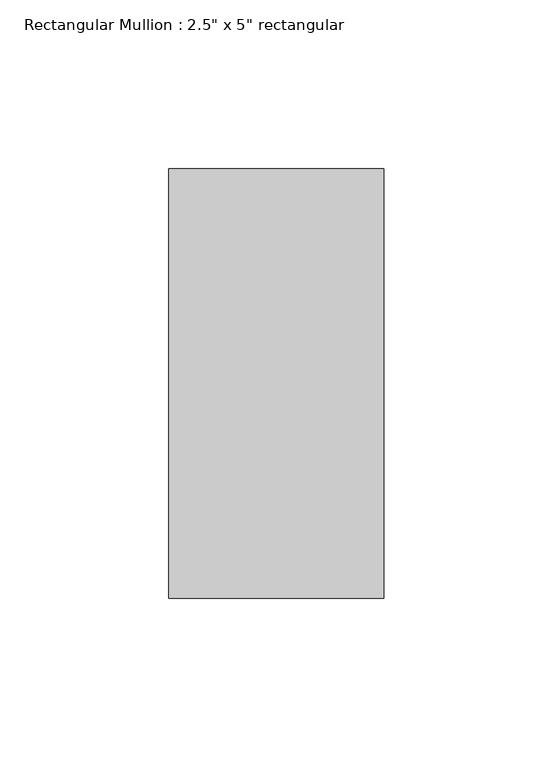
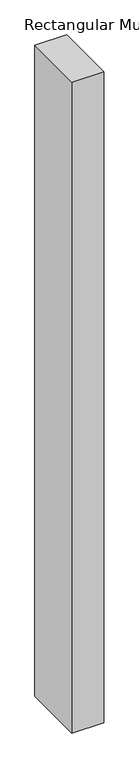
"""IFC4 building model written with IfcOpenShell, lengths in millimetres: member geometry."""

from ifc_helpers import new_model, si_unit, frame, origin, place, context, project, spatial, polyline, outline, extrude, source, transform, mapped, element, save


def member_30211588(model_context):
    return source(origin(), model_context, "Body", "SweptSolid", [
        extrude(outline(polyline([(31.75, 63.5), (31.75, -63.5), (-31.75, -63.5), (-31.75, 63.5), (31.75, 63.5)])), frame((0.0, 0.0, -1367.3666665), z_axis=(0.0, 0.0, 1.0), x_axis=(1.0, 0.0, 0.0)), (0.0, 0.0, 1.0), 1367.3666665),
    ])


if __name__ == "__main__":
    model = new_model("IFC4")
    model_context = context("Model", 3, world=origin())
    ifc_project = project(units=[si_unit("LENGTHUNIT", "METRE", prefix="MILLI")], contexts=[model_context])
    site = spatial("IfcSite", under=ifc_project)
    building = spatial("IfcBuilding", under=site)
    placement = place(None, origin())
    member_shape = member_30211588(model_context)
    element("IfcMember", 1, ObjectType="Rectangular Mullion : 2.5\" x 5\" rectangular", at=placement, inside=building, context=model_context, shape_type="MappedRepresentation", body=[
        mapped(member_shape, transform((0.0, 0.0, 0.0), x_axis=(1.0, 0.0, 0.0), y_axis=(0.0, 1.0, 0.0), z_axis=(0.0, 0.0, 1.0))),
    ])
    save(model, "model.ifc")

# Revit data of these elements
# Type "Rectangular Mullion : 2.5\" x 5\" rectangular"
#   built-in parameter 1007304 = 0.416667 (stored number, unit not read)
#   built-in parameter 1007301 = 0.104167 (stored number, unit not read)
#   built-in parameter 1007300 = 0.104167 (stored number, unit not read)
# Element 1 (IfcMember, "Rectangular Mullion : 2.5\" x 5\" rectangular")
#   Materials on its faces: "Aluminum"
# Materials
#   "Aluminum": class "Metal", colour RGB 247 247 247, transparency 0, Description = "Aluminum 6061", Cost = 0
